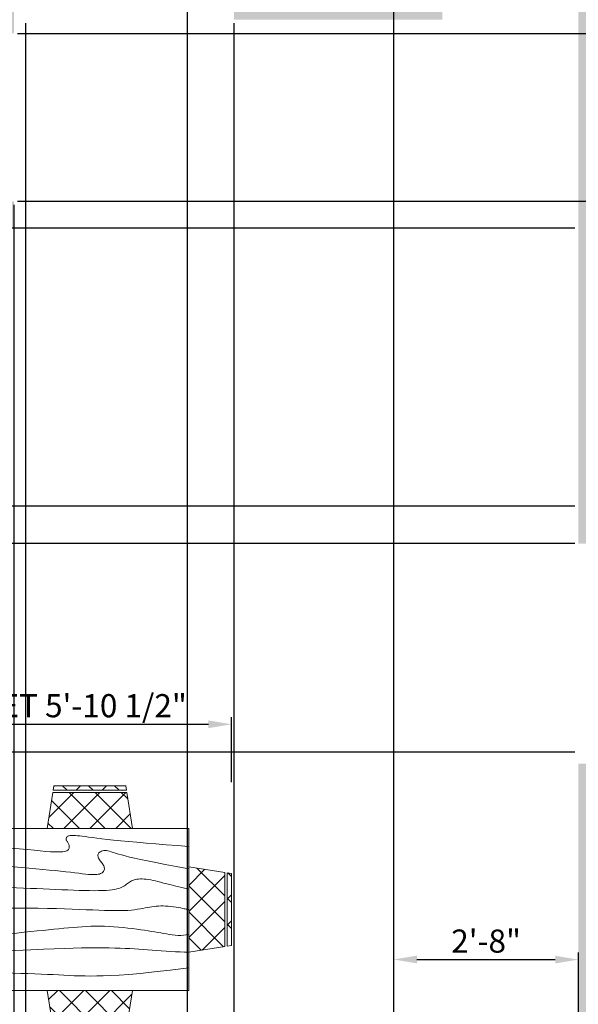
# Model space of a CAD drawing. Units: inches. Extents: x 1872 to 2380, y 714 to 1327.
# Tile 7 of 9: x 2101 to 2198, y 974 to 1144. Entities that reach past the tile are written whole.
import ezdxf

# ---------------------------------------------------------------- set-up
doc = ezdxf.new("R2010")
doc.units = ezdxf.units.IN
doc.layers.add('A-ANNO-DIMS', color=2, linetype='Continuous', lineweight=18)
doc.layers.add('A-FURN', color=8, linetype='Continuous', lineweight=18)
doc.layers.add('A-FURN-PATT', color=254, linetype='Continuous', lineweight=13, true_color=0xf8ceb3)
doc.layers.add('A-WALL-PATT', color=242, linetype='Continuous', lineweight=13, true_color=0xd52e31)
doc.styles.get("Standard").update_dxf_attribs({"font": 'arial.ttf'})
doc.dimstyles.new('ISO-25', dxfattribs={"dimtxt": 4, "dimasz": 4, "dimexe": 1.25, "dimexo": 0.625, "dimtad": 1, "dimdec": 0, "dimlunit": 3, "dimtxsty": 'Standard', "dimcen": 2.5, "dimadec": 0, "dimazin": 0, "dimtfac": 1, "dimtdec": 0, "dimtmove": 0, "dimatfit": 3, "dimfxl": 1, "dimarcsym": 0})

# ---------------------------------------------------------------- blocks, each defined once
blk = doc.blocks.new('Dining Set - 36 x 72 in.')
for p, q in [((-22, 27.5), (-22.1562, 26.50042)), ((-5.8416, 26.5), (-22.1534, 26.5)), ((-22, 27.5), (-6, 27.5)), ((-5.8437, 26.49966), (-6, 27.5)), ((6, 27.5), (5.8438, 26.50042)), ((22.1584, 26.5), (5.8466, 26.5)), ((6, 27.5), (22, 27.5)), ((22.1563, 26.49966), (22, 27.5)), ((-22.2343, 26.00059), (-23.4847, 17.99762)), ((-22.2304, 26), (-5.7608, 26)), ((-4.5152, 17.99762), (-5.7655, 25.99926)), ((5.7657, 26.00059), (4.5153, 17.99762)), ((5.7696, 26), (22.2392, 26)), ((23.4848, 17.99762), (22.2345, 25.99926)), ((36, 18), (-36, 18)), ((-36, 18), (-36, -18)), ((36, -18), (36, 18)), ((-44.0006, 8.23428), (-35.9976, 9.48474)), ((44.0006, 8.23428), (35.9976, 9.48474)), ((-45.5, 8), (-44.5004, 8.15617)), ((-45.5, 8), (-45.5, -8)), ((-44.5, -8.15843), (-44.5, 8.15338)), ((-44, 8.23041), (-44, -8.23915)), ((44, 8.23041), (44, -8.23915)), ((44.5, -8.15843), (44.5, 8.15338)), ((45.5, 8), (44.5005, 8.15617)), ((45.5, 8), (45.5, -8)), ((-44.4997, -8.15631), (-45.5, -8)), ((-35.9976, -9.48476), (-43.9993, -8.2345)), ((35.9976, -9.48476), (43.9993, -8.2345)), ((44.4997, -8.15631), (45.5, -8)), ((-36, -18), (36, -18)), ((-22.2343, -26.0006), (-23.4847, -17.99762)), ((-4.5152, -17.99762), (-5.7655, -25.99928)), ((5.7657, -26.0006), (4.5153, -17.99762)), ((23.4848, -17.99762), (22.2345, -25.99928)), ((-22.2304, -26), (-5.7608, -26)), ((5.7696, -26), (22.2392, -26)), ((-22, -27.5), (-22.1562, -26.50044)), ((-5.8416, -26.5), (-22.1534, -26.5)), ((-22, -27.5), (-6, -27.5)), ((-5.8437, -26.49967), (-6, -27.5)), ((6, -27.5), (5.8438, -26.50044)), ((22.1584, -26.5), (5.8466, -26.5)), ((6, -27.5), (22, -27.5)), ((22.1563, -26.49967), (22, -27.5))]:
    blk.add_line(p, q)
for points in [[(-36, 15), (-31.1772, 14.97754), (-26.8079, 14.91406), (-22.8538, 14.81543), (-19.276, 14.6875), (-16.0362, 14.53613), (-13.0957, 14.36718), (-10.4159, 14.18652), (-7.9583, 14), (-5.6904, 13.81315), (-3.6035, 13.63021), (-1.6954, 13.45508), (0.0365, 13.29166), (1.5945, 13.14388), (2.9811, 13.01562), (4.1988, 12.9108), (5.25, 12.83333), (6.1393, 12.78613), (6.8802, 12.76823), (7.4883, 12.77767), (7.9792, 12.8125), (8.3685, 12.87077), (8.6719, 12.95052), (8.9049, 13.0498), (9.0833, 13.16666), (9.2205, 13.29899), (9.3216, 13.44401), (9.3895, 13.59879), (9.4271, 13.76041), (9.4373, 13.92594), (9.4232, 14.09245), (9.3875, 14.257), (9.3333, 14.41666), (9.2638, 14.56917), (9.1836, 14.71484), (9.0975, 14.85465), (9.0104, 14.98958), (8.9272, 15.1206), (8.8529, 15.2487), (8.7922, 15.37483), (8.75, 15.5), (8.7305, 15.62467), (8.7344, 15.74739), (8.7617, 15.86621), (8.8125, 15.97916), (8.8867, 16.08431), (8.9844, 16.17968), (9.1055, 16.26334), (9.25, 16.33333), (9.4189, 16.38802), (9.6172, 16.42708), (9.8506, 16.45052), (10.125, 16.45833), (10.4463, 16.45052), (10.8203, 16.42708), (11.2529, 16.38802), (11.75, 16.33333), (12.3184, 16.26318), (12.9694, 16.17838), (13.7151, 16.07991), (14.5677, 15.96875), (15.5395, 15.84586), (16.6426, 15.71224), (17.8893, 15.56884), (19.2917, 15.41666), (20.859, 15.25667), (22.5879, 15.08984), (24.4721, 14.91715), (26.5052, 14.73958), (28.6809, 14.5581), (30.9929, 14.3737), (33.4347, 14.18733), (36, 14)], [(-36, 10), (-28.9766, 10.14274), (-23.1725, 10.20442), (-18.4241, 10.19775), (-14.5677, 10.13541), (-11.4399, 10.03011), (-8.877, 9.89453), (-6.7154, 9.74137), (-4.7917, 9.58333), (-2.9698, 9.43082), (-1.2246, 9.28515), (0.4415, 9.14534), (2.026, 9.01041), (3.5266, 8.87939), (4.9408, 8.7513), (6.266, 8.62516), (7.5, 8.5), (8.6411, 8.37549), (9.6914, 8.2539), (10.6538, 8.13818), (11.5312, 8.03125), (12.3267, 7.93603), (13.043, 7.85547), (13.6831, 7.79248), (14.25, 7.75), (14.7471, 7.7303), (15.1797, 7.73307), (15.5537, 7.75732), (15.875, 7.80208), (16.1494, 7.86637), (16.3828, 7.94922), (16.5811, 8.04964), (16.75, 8.16666), (16.8944, 8.29915), (17.0143, 8.44531), (17.1089, 8.60319), (17.1771, 8.77083), (17.218, 8.94629), (17.2305, 9.1276), (17.2137, 9.31282), (17.1667, 9.5), (17.0895, 9.6875), (16.987, 9.875), (16.8649, 10.0625), (16.7292, 10.25), (16.5856, 10.4375), (16.4401, 10.625), (16.2985, 10.8125), (16.1667, 11), (16.05, 11.18733), (15.9518, 11.3737), (15.8752, 11.5581), (15.8229, 11.73958), (15.798, 11.91715), (15.8034, 12.08984), (15.842, 12.25667), (15.9167, 12.41666), (16.0295, 12.56836), (16.1784, 12.70833), (16.3605, 12.83268), (16.5729, 12.9375), (16.8127, 13.01888), (17.0768, 13.07291), (17.3625, 13.0957), (17.6667, 13.08333), (17.9894, 13.03312), (18.3418, 12.94726), (18.7382, 12.82918), (19.1927, 12.68229), (19.7195, 12.51001), (20.3327, 12.31575), (21.0465, 12.10294), (21.875, 11.875), (22.8357, 11.63354), (23.959, 11.37304), (25.2786, 11.08618), (26.8282, 10.76562), (28.6414, 10.40405), (30.752, 9.99414), (33.1936, 9.52856), (36, 9)], [(-36, 5.5), (-30.7157, 5.3348), (-26.069, 5.20963), (-21.9946, 5.11767), (-18.4271, 5.05208), (-15.3009, 5.00602), (-12.5508, 4.97265), (-10.1112, 4.94515), (-7.9167, 4.91666), (-5.909, 4.88167), (-4.0586, 4.83984), (-2.3429, 4.79215), (-0.7396, 4.73958), (0.7739, 4.6831), (2.22, 4.6237), (3.6213, 4.56233), (5, 4.5), (6.373, 4.43782), (7.7344, 4.3776), (9.0723, 4.32129), (10.375, 4.27083), (11.6309, 4.22819), (12.8281, 4.19531), (13.9551, 4.17415), (15, 4.16666), (15.954, 4.17448), (16.819, 4.19791), (17.6001, 4.23698), (18.3021, 4.29166), (18.9299, 4.36198), (19.4883, 4.44791), (19.9823, 4.54948), (20.4167, 4.66666), (20.7969, 4.79899), (21.1302, 4.94401), (21.4245, 5.09879), (21.6875, 5.26041), (21.9271, 5.42594), (22.1511, 5.59245), (22.3672, 5.757), (22.5834, 5.91666), (22.8065, 6.06868), (23.0404, 6.21093), (23.2879, 6.34147), (23.5521, 6.45833), (23.8358, 6.55957), (24.142, 6.64323), (24.4735, 6.70735), (24.8334, 6.75), (25.2235, 6.76969), (25.642, 6.76692), (26.0858, 6.74267), (26.5521, 6.69791), (27.0379, 6.63362), (27.5404, 6.55078), (28.0565, 6.45036), (28.5834, 6.33333), (29.1242, 6.19987), (29.7071, 6.04687), (30.3661, 5.87044), (31.1354, 5.66666), (32.0493, 5.43164), (33.142, 5.16146), (34.4475, 4.85221), (36, 4.5)], [(-36, -1), (-30.7915, -0.6591), (-26.0195, -0.38216), (-21.6519, -0.16284), (-17.6563, 0.00521), (-14.0005, 0.12833), (-10.6523, 0.21289), (-7.5796, 0.26522), (-4.75, 0.29166), (-2.134, 0.29793), (0.2878, 0.28711), (2.5317, 0.26163), (4.6146, 0.22396), (6.5529, 0.17651), (8.3633, 0.12174), (10.0623, 0.06209), (11.6667, 0), (13.1899, -0.06201), (14.6341, -0.1211), (15.9982, -0.17432), (17.2813, -0.21875), (18.4823, -0.25147), (19.6003, -0.26953), (20.6343, -0.27002), (21.5834, -0.25), (22.4481, -0.20768), (23.2357, -0.14584), (23.9549, -0.06836), (24.6146, 0.02083), (25.2235, 0.11784), (25.7904, 0.21875), (26.3241, 0.31966), (26.8334, 0.41666), (27.3265, 0.50618), (27.8099, 0.58593), (28.2894, 0.65397), (28.7709, 0.70833), (29.2601, 0.74707), (29.763, 0.76823), (30.2855, 0.76985), (30.8334, 0.75), (31.4088, 0.70784), (31.9994, 0.64713), (32.589, 0.57275), (33.1615, 0.48958), (33.7008, 0.4025), (34.1908, 0.3164), (34.6153, 0.23616), (34.9584, 0.16666), (35.2099, 0.11165), (35.3848, 0.07031), (35.504, 0.04069), (35.5886, 0.02083), (35.6594, 0.00879), (35.7377, 0.0026), (35.8442, 0.00032), (36, 0)], [(-36, -6.5), (-27.1843, -6.31267), (-20.084, -6.1263), (-14.469, -5.9419), (-10.1094, -5.76042), (-6.7752, -5.58285), (-4.2363, -5.41016), (-2.2629, -5.24333), (-0.625, -5.08334), (0.8708, -4.93099), (2.2715, -4.78646), (3.5872, -4.64974), (4.8281, -4.52084), (6.0046, -4.39974), (7.127, -4.28646), (8.2053, -4.18099), (9.25, -4.08334), (10.2705, -3.99382), (11.2734, -3.91407), (12.2647, -3.84603), (13.25, -3.79167), (14.2354, -3.75293), (15.2266, -3.73177), (16.2295, -3.73015), (17.25, -3.75), (18.2912, -3.79248), (19.3451, -3.85547), (20.4009, -3.93604), (21.4479, -4.03125), (22.4754, -4.13819), (23.4727, -4.25391), (24.4289, -4.37549), (25.3334, -4.5), (26.1785, -4.62492), (26.9694, -4.74935), (27.7145, -4.87281), (28.4219, -4.99479), (29.1, -5.11483), (29.7572, -5.23242), (30.4016, -5.34709), (31.0417, -5.45834), (31.6837, -5.56437), (32.3262, -5.65821), (32.9658, -5.73153), (33.599, -5.77604), (34.2224, -5.78345), (34.8327, -5.74545), (35.4264, -5.65373), (36, -5.5)], [(-36, -10), (-26.4022, -9.81299), (-18.4675, -9.62891), (-11.9839, -9.45069), (-6.7396, -9.28125), (-2.5226, -9.12354), (0.8789, -8.98047), (3.6769, -8.85498), (6.0833, -8.75), (8.2767, -8.66765), (10.3021, -8.60677), (12.1712, -8.56543), (13.8958, -8.54167), (15.4876, -8.53353), (16.9583, -8.53907), (18.3197, -8.55632), (19.5834, -8.58334), (20.7616, -8.61841), (21.8685, -8.66081), (22.9188, -8.71004), (23.9271, -8.76563), (24.9081, -8.82707), (25.8763, -8.89388), (26.8465, -8.96558), (27.8334, -9.04167), (28.8474, -9.12118), (29.8828, -9.20117), (30.93, -9.27824), (31.9792, -9.34896), (33.0205, -9.40991), (34.0443, -9.45768), (35.0407, -9.48885), (36, -9.5)], [(-36, -14.5), (-30.0881, -14.33513), (-25.0332, -14.21224), (-20.7312, -14.12647), (-17.0781, -14.07292), (-13.97, -14.04671), (-11.3027, -14.04297), (-8.9724, -14.05681), (-6.875, -14.08334), (-4.9224, -14.11833), (-3.0905, -14.16016), (-1.3709, -14.20785), (0.2448, -14.26042), (1.7647, -14.3169), (3.1973, -14.3763), (4.5507, -14.43767), (5.8333, -14.5), (7.0554, -14.5621), (8.235, -14.62175), (9.3922, -14.67652), (10.5469, -14.72396), (11.7192, -14.76164), (12.929, -14.78711), (14.1965, -14.79794), (15.5417, -14.79167), (16.9933, -14.76424), (18.6152, -14.70508), (20.4804, -14.60197), (22.6615, -14.44271), (25.2312, -14.21509), (28.2624, -13.9069), (31.8277, -13.50594), (36, -13)]]:
    blk.add_lwpolyline(points)
blk = doc.blocks.new('*D46')
at = {"layer": 'A-ANNO-DIMS', "color": 0, "lineweight": -2, "transparency": 16777216}
for p, q in [((2067.28, 1012.46), (2067.28, 1023.69)), ((2071.28, 1022.44), (2133.99, 1022.44)), ((2137.99, 1012.46), (2137.99, 1023.69))]:
    blk.add_line(p, q, dxfattribs=at)
at = {"layer": 'A-ANNO-DIMS', "color": 0, "transparency": 16777216}
for points in [[(2071.28, 1023.11), (2071.28, 1021.77), (2067.28, 1022.44)], [(2133.99, 1023.11), (2133.99, 1021.77), (2137.99, 1022.44)]]:
    blk.add_solid(points, dxfattribs=at)
at = {"layer": 'Defpoints', "color": 0, "transparency": 16777216}
for p in [(2137.99, 1022.44), (2067.28, 1011.83), (2137.99, 1011.83)]:
    blk.add_point(p, dxfattribs=at)
at = {"layer": 'A-ANNO-DIMS', "color": 0, "transparency": 16777216, "insert": (2102.64, 1025.13), "char_height": 4, "attachment_point": 5}
blk.add_mtext('DINING SET 5\'-10 1/2"', dxfattribs=at)
blk = doc.blocks.new('*D69')
at = {"layer": 'A-ANNO-DIMS', "color": 0, "lineweight": -2, "transparency": 16777216}
for p, q in [((2101.02, 1141.77), (2377.6, 1141.77)), ((2376.35, 1116.77), (2376.35, 1137.77)), ((2101.02, 1112.77), (2377.6, 1112.77))]:
    blk.add_line(p, q, dxfattribs=at)
at = {"layer": 'A-ANNO-DIMS', "color": 0, "transparency": 16777216}
for points in [[(2375.68, 1137.77), (2377.01, 1137.77), (2376.35, 1141.77)], [(2375.68, 1116.77), (2377.01, 1116.77), (2376.35, 1112.77)]]:
    blk.add_solid(points, dxfattribs=at)
at = {"layer": 'Defpoints', "color": 0, "transparency": 16777216}
for p in [(2100.4, 1141.77), (2376.35, 1141.77), (2100.4, 1112.77)]:
    blk.add_point(p, dxfattribs=at)
at = {"layer": 'A-ANNO-DIMS', "color": 0, "transparency": 16777216, "insert": (2373.68, 1127.27), "char_height": 4, "attachment_point": 5, "rotation": 90}
blk.add_mtext('2\'-5"', dxfattribs=at)
blk = doc.blocks.new('*D70')
at = {"layer": 'A-ANNO-DIMS', "color": 0, "lineweight": -2, "transparency": 16777216}
for p, q in [((2102.4, 1143.52), (2102.4, 716.39)), ((2138.4, 1143.52), (2138.4, 716.39)), ((2106.4, 717.64), (2134.4, 717.64))]:
    blk.add_line(p, q, dxfattribs=at)
at = {"layer": 'A-ANNO-DIMS', "color": 0, "transparency": 16777216}
for points in [[(2106.4, 718.3), (2106.4, 716.97), (2102.4, 717.64)], [(2134.4, 718.3), (2134.4, 716.97), (2138.4, 717.64)]]:
    blk.add_solid(points, dxfattribs=at)
at = {"layer": 'Defpoints', "color": 0, "transparency": 16777216}
for p in [(2102.4, 1144.14), (2138.4, 1144.14), (2138.4, 717.64)]:
    blk.add_point(p, dxfattribs=at)
at = {"layer": 'A-ANNO-DIMS', "color": 0, "transparency": 16777216, "insert": (2120.4, 720.31), "char_height": 4, "attachment_point": 5}
blk.add_mtext('3\'-0"', dxfattribs=at)
blk = doc.blocks.new('*D72')
at = {"layer": 'A-ANNO-DIMS', "color": 0, "lineweight": -2, "transparency": 16777216}
for p, q in [((2197.27, 1108.14), (1905.35, 1108.14)), ((1906.6, 1064.14), (1906.6, 1104.14)), ((2197.27, 1060.14), (1905.35, 1060.14))]:
    blk.add_line(p, q, dxfattribs=at)
at = {"layer": 'A-ANNO-DIMS', "color": 0, "transparency": 16777216}
for points in [[(1905.93, 1104.14), (1907.27, 1104.14), (1906.6, 1108.14)], [(1905.93, 1064.14), (1907.27, 1064.14), (1906.6, 1060.14)]]:
    blk.add_solid(points, dxfattribs=at)
at = {"layer": 'Defpoints', "color": 0, "transparency": 16777216}
for p in [(1906.6, 1108.14), (2197.9, 1108.14), (2197.9, 1060.14)]:
    blk.add_point(p, dxfattribs=at)
at = {"layer": 'A-ANNO-DIMS', "color": 0, "transparency": 16777216, "insert": (1903.93, 1084.14), "char_height": 4, "attachment_point": 5, "rotation": 90}
blk.add_mtext('4\'-0"', dxfattribs=at)
blk = doc.blocks.new('*D73')
at = {"layer": 'A-ANNO-DIMS', "color": 0, "lineweight": -2, "transparency": 16777216}
for p, q in [((2197.27, 1053.64), (1905.35, 1053.64)), ((1906.6, 1021.64), (1906.6, 1049.64)), ((2197.27, 1017.64), (1905.35, 1017.64))]:
    blk.add_line(p, q, dxfattribs=at)
at = {"layer": 'A-ANNO-DIMS', "color": 0, "transparency": 16777216}
for points in [[(1905.93, 1049.64), (1907.27, 1049.64), (1906.6, 1053.64)], [(1905.93, 1021.64), (1907.27, 1021.64), (1906.6, 1017.64)]]:
    blk.add_solid(points, dxfattribs=at)
at = {"layer": 'Defpoints', "color": 0, "transparency": 16777216}
for p in [(1906.6, 1053.64), (2197.9, 1053.64), (2197.9, 1017.64)]:
    blk.add_point(p, dxfattribs=at)
at = {"layer": 'A-ANNO-DIMS', "color": 0, "transparency": 16777216, "insert": (1903.93, 1035.64), "char_height": 4, "attachment_point": 5, "rotation": 90}
blk.add_mtext('3\'-0"', dxfattribs=at)
blk = doc.blocks.new('*D74')
at = {"layer": 'A-ANNO-DIMS', "color": 0, "lineweight": -2, "transparency": 16777216}
for p, q in [((2130.4, 953.62), (2130.4, 1319.69)), ((2134.4, 1318.44), (2162.01, 1318.44)), ((2166.01, 953.64), (2166.01, 1319.69))]:
    blk.add_line(p, q, dxfattribs=at)
at = {"layer": 'A-ANNO-DIMS', "color": 0, "transparency": 16777216}
for points in [[(2134.4, 1319.11), (2134.4, 1317.78), (2130.4, 1318.44)], [(2162.01, 1319.11), (2162.01, 1317.78), (2166.01, 1318.44)]]:
    blk.add_solid(points, dxfattribs=at)
at = {"layer": 'Defpoints', "color": 0, "transparency": 16777216}
for p in [(2166.01, 1318.44), (2130.4, 952.99), (2166.01, 953.01)]:
    blk.add_point(p, dxfattribs=at)
at = {"layer": 'A-ANNO-DIMS', "color": 0, "transparency": 16777216, "insert": (2148.2, 1321.14), "char_height": 4, "attachment_point": 5}
blk.add_mtext('2\'-11 1/2"', dxfattribs=at)
blk = doc.blocks.new('*D75')
at = {"layer": 'A-ANNO-DIMS', "color": 0, "lineweight": -2, "transparency": 16777216}
for p, q in [((2166.01, 953.64), (2166.02, 983.06)), ((2197.9, 953.62), (2197.91, 983.04)), ((2170.02, 981.81), (2193.91, 981.8))]:
    blk.add_line(p, q, dxfattribs=at)
at = {"layer": 'A-ANNO-DIMS', "color": 0, "transparency": 16777216}
for points in [[(2170.02, 982.48), (2170.02, 981.14), (2166.02, 981.81)], [(2193.91, 982.46), (2193.91, 981.13), (2197.91, 981.79)]]:
    blk.add_solid(points, dxfattribs=at)
at = {"layer": 'Defpoints', "color": 0, "transparency": 16777216}
for p in [(2197.91, 981.79), (2166.01, 953.01), (2197.9, 952.99)]:
    blk.add_point(p, dxfattribs=at)
at = {"layer": 'A-ANNO-DIMS', "color": 0, "transparency": 16777216, "insert": (2181.97, 984.47), "char_height": 4, "attachment_point": 5, "rotation": 359.9714}
blk.add_mtext('2\'-8"', dxfattribs=at)
blk = doc.blocks.new('*D80')
at = {"layer": 'A-ANNO-DIMS', "color": 0, "lineweight": -2, "transparency": 16777216}
for p, q in [((2095.9, 1112.15), (2095.9, 716.39)), ((2100.4, 1112.15), (2100.4, 716.39)), ((2091.9, 717.64), (2087.9, 717.64)), ((2095.9, 717.64), (2100.4, 717.64)), ((2104.4, 717.64), (2129.6, 717.64))]:
    blk.add_line(p, q, dxfattribs=at)
at = {"layer": 'A-ANNO-DIMS', "color": 0, "transparency": 16777216}
for points in [[(2091.9, 718.3), (2091.9, 716.97), (2095.9, 717.64)], [(2104.4, 718.3), (2104.4, 716.97), (2100.4, 717.64)]]:
    blk.add_solid(points, dxfattribs=at)
at = {"layer": 'Defpoints', "color": 0, "transparency": 16777216}
for p in [(2095.9, 1112.77), (2100.4, 1112.77), (2100.4, 717.64)]:
    blk.add_point(p, dxfattribs=at)
at = {"layer": 'A-ANNO-DIMS', "color": 0, "transparency": 16777216, "insert": (2119, 720.33), "char_height": 4, "attachment_point": 5}
blk.add_mtext('0\'-4 1/2"', dxfattribs=at)

msp = doc.modelspace()

# ---------------------------------------------------------------- hatches: boundary and pattern name
at = {"layer": 'A-FURN-PATT', "transparency": 33554687}
h = msp.add_hatch(dxfattribs=at)
h.set_pattern_fill('ANSI37', color=256)
h.paths.add_polyline_path([(2030.37, 1262.04), (1979.97, 1262.04), (1979.97, 1246.84), (1967.17, 1246.84), (1967.17, 1202.04), (2030.37, 1202.04)])
h.paths.add_polyline_path([(1964.77, 1246.84), (1966.77, 1248.84), (1966.77, 1254.04), (1951.57, 1254.04), (1951.57, 1233.24), (1964.77, 1233.24)])
h.paths.add_polyline_path([(1964.77, 1230.84), (1951.57, 1230.84), (1951.57, 1210.04), (1964.77, 1210.04)])
h.paths.add_polyline_path([(2268.08, 1263.68), (2221.12, 1263.68), (2221.12, 1219.09), (2258.57, 1219.09), (2258.57, 1230.39), (2268.08, 1230.39)])
h.paths.add_polyline_path([(2279.67, 1257.73), (2269.86, 1257.73), (2269.86, 1242.28), (2279.67, 1242.28)])
h.paths.add_polyline_path([(2279.67, 1240.49), (2269.86, 1240.49), (2269.86, 1230.39), (2268.38, 1228.9), (2268.38, 1225.04), (2279.67, 1225.04)])
h.paths.add_polyline_path([(2097.97, 1011.83), (2085.54, 1011.83), (2085.42, 1011.06), (2098.09, 1011.06)])
h.paths.add_polyline_path([(2098.15, 1010.67), (2085.36, 1010.67), (2084.39, 1004.45), (2099.13, 1004.45)])
h.paths.add_polyline_path([(2119.91, 1010.67), (2107.12, 1010.67), (2106.14, 1004.45), (2120.89, 1004.45)])
h.paths.add_polyline_path([(2119.73, 1011.83), (2107.3, 1011.83), (2107.18, 1011.06), (2119.85, 1011.06)])
h.paths.add_polyline_path([(2074.66, 997.83), (2068.44, 996.86), (2068.44, 984.06), (2074.66, 983.09)])
h.paths.add_polyline_path([(2068.05, 996.8), (2067.28, 996.68), (2067.28, 984.25), (2068.05, 984.12)])
h.paths.add_polyline_path([(2136.83, 996.86), (2130.61, 997.83), (2130.61, 983.09), (2136.83, 984.06)])
h.paths.add_polyline_path([(2137.99, 996.68), (2137.22, 996.8), (2137.22, 984.12), (2137.99, 984.25)])
h.paths.add_polyline_path([(2099.13, 976.47), (2084.39, 976.47), (2085.36, 970.26), (2098.15, 970.26)])
h.paths.add_polyline_path([(2120.89, 976.47), (2106.14, 976.47), (2107.12, 970.26), (2119.91, 970.26)])
h.paths.add_polyline_path([(2119.85, 969.87), (2107.18, 969.87), (2107.3, 969.09), (2119.73, 969.09)])
h.paths.add_polyline_path([(2098.09, 969.87), (2085.42, 969.87), (2085.54, 969.09), (2097.97, 969.09)])
at = {"layer": 'A-WALL-PATT', "transparency": 33554687}
h = msp.add_hatch(color=256, dxfattribs=at)
h.dxf.hatch_style = 1
h.paths.add_polyline_path([(2295.4, 1289.64), (1935.4, 1289.64), (1935.4, 809.64), (1949.4, 809.64), (1949.4, 818.64), (1944.4, 818.64), (1944.4, 1108.27), (2100.4, 1108.27), (2100.4, 1112.77), (1944.4, 1112.77), (1944.4, 1280.64), (2095.9, 1280.64), (2095.9, 1141.77), (2100.4, 1141.77), (2100.4, 1280.64), (2169.91, 1280.64), (2169.91, 1244.64), (2169.91, 1160.49, -0.053008), (2170.04, 1158.75, -0.03687), (2169.91, 1157.54), (2169.91, 1148.64), (2167.91, 1148.64), (2138.4, 1148.64), (2138.4, 1144.14), (2167.91, 1144.14), (2174.41, 1144.14), (2174.41, 1280.64), (2197.9, 1280.64), (2197.9, 1184.64), (2202.4, 1184.64), (2202.4, 1280.64), (2286.4, 1280.64), (2286.4, 1148.64), (2197.9, 1148.64), (2197.9, 1108.14), (2202.4, 1108.14), (2202.4, 1144.14), (2286.4, 1144.14), (2286.4, 1060.14), (2202.4, 1060.14), (2202.4, 1108.14), (2197.9, 1108.14), (2197.9, 1060.14), (2197.9, 1053.64), (2202.4, 1053.64), (2202.4, 1055.64), (2286.4, 1055.64), (2286.4, 976.14), (2202.4, 976.14), (2202.4, 1015.64), (2197.9, 1015.64), (2197.9, 971.64), (2197.9, 952.99), (2197.9, 818.64), (2101.9, 818.64), (2101.9, 948.71), (2130.4, 948.71), (2130.4, 952.99), (2073.4, 952.99), (2073.4, 948.71), (2097.4, 948.71), (2097.4, 818.64), (2005.9, 818.64), (2005.9, 948.71), (2029.9, 948.71), (2029.9, 952.99), (2001.4, 952.99), (2001.4, 818.64), (1996.4, 818.64), (1985.23, 818.64), (1985.23, 809.64), (1996.4, 809.64), (2295.4, 809.64)])
h.paths.add_polyline_path([(2202.4, 971.64), (2286.4, 971.64), (2286.4, 858.19), (2286.62, 858.19), (2286.62, 857.19), (2286.4, 857.19), (2286.4, 828.68), (2286.48, 828.76), (2286.4, 828.43), (2286.4, 818.64), (2256.29, 818.64), (2255.29, 818.39), (2254.54, 818.64), (2238.99, 818.64), (2238.75, 818.58), (2238.56, 818.64), (2202.4, 818.64), (2202.4, 952.99)], flags=16)
h.paths.add_polyline_path([(2260.41, 970, -0.15), (2280.41, 970), (2278.41, 967, 0.001913), (2277.92, 967.06), (2277.41, 964.5), (2278.64, 964.5), (2278.72, 964), (2279.41, 964), (2282.41, 953, -0.541163), (2280.76, 950.93), (2280.91, 950, -0.414214), (2279.91, 949), (2279.41, 949), (2279.91, 945), (2278.41, 945), (2277.91, 949), (2270.41, 949), (2262.91, 949), (2262.41, 945), (2260.91, 945), (2261.41, 949), (2260.91, 949, -0.414214), (2259.91, 950), (2260.05, 950.93, -0.505809), (2258.36, 952.83), (2261.41, 964), (2262.1, 964), (2262.17, 964.5), (2263.41, 964.5), (2262.9, 967.06, 0.001913), (2262.41, 967)], flags=0)
h.paths.add_polyline_path([(2257.85, 934.42), (2280.51, 934.42, -0.333333), (2281.77, 933.16), (2281.77, 923.09, -0.333333), (2280.51, 921.83), (2277.57, 921.83), (2277.57, 921.41), (2275.89, 921.41), (2275.89, 921.83), (2262.46, 921.83), (2262.46, 921.41), (2260.79, 921.41), (2260.79, 921.83), (2257.85, 921.83, -0.333333), (2256.59, 923.09), (2256.59, 933.16, -0.333333)], flags=0)
h.paths.add_polyline_path([(2260.61, 912.79), (2262.11, 912.79), (2262.61, 908.79), (2270.11, 908.79), (2277.61, 908.79), (2278.11, 912.79), (2279.61, 912.79), (2279.11, 908.79), (2279.61, 908.79, -0.414214), (2280.61, 907.79), (2280.46, 906.86, -0.505809), (2282.15, 904.96), (2279.11, 893.79), (2278.42, 893.79), (2278.34, 893.29), (2277.11, 893.29), (2277.62, 890.73, 0.001913), (2278.11, 890.79), (2280.11, 887.79, -0.15), (2260.11, 887.79), (2262.11, 890.79, 0.001913), (2262.59, 890.73), (2263.11, 893.29), (2261.87, 893.29), (2261.79, 893.79), (2261.11, 893.79), (2258.11, 904.79, -0.541163), (2259.75, 906.86), (2259.61, 907.79, -0.414214), (2260.61, 908.79), (2261.11, 908.79)], flags=0)
h.paths.add_polyline_path([(2252.62, 864.69), (2253.62, 864.69), (2253.62, 862.19), (2253.62, 860.69), (2256.62, 859.69, -0.362186), (2259.62, 862.19, -0.174416), (2262.62, 860.69, 0.103487), (2265.62, 859.19, -0.219276), (2266.55, 858.19), (2268.62, 858.19), (2268.62, 859.69), (2267.62, 859.69), (2267.62, 863.69), (2270.12, 863.69), (2270.12, 859.69), (2269.12, 859.69), (2269.12, 858.19), (2274.62, 858.19), (2278.62, 858.19), (2278.62, 862.69), (2275.62, 864.69), (2275.62, 865.69), (2279.62, 862.69), (2279.62, 858.19), (2279.62, 852.69), (2275.62, 849.19), (2275.62, 850.19), (2278.62, 852.69), (2278.62, 857.19), (2274.62, 857.19), (2271.12, 857.19), (2271.12, 855.69), (2272.12, 855.69), (2272.12, 851.69), (2269.62, 851.69), (2269.62, 855.69), (2270.62, 855.69), (2270.62, 857.19), (2266.55, 857.19, -0.219162), (2265.62, 856.19, 0.103506), (2262.62, 854.69, -0.174459), (2259.62, 853.19, -0.362114), (2256.62, 855.69), (2253.62, 854.69), (2253.62, 850.69), (2252.62, 850.69)], flags=0)
h.paths.add_polyline_path([(2253.62, 859.69), (2256.62, 858.69), (2256.62, 856.69), (2253.62, 855.69)], flags=0)
h.paths.add_polyline_path([(2208.62, 838.17), (2208.28, 836.61), (2207.75, 836.18), (2207.67, 833.93), (2208.71, 832.96), (2211.55, 836.09), (2214.43, 837.53), (2214.45, 837.55), (2214.61, 836.16), (2215.48, 834.9), (2215.87, 835.13), (2217.12, 836.79), (2216.83, 834.17), (2218.8, 828.76), (2219.23, 829.13), (2220.06, 831.53), (2219.5, 837.61), (2219.53, 837.66), (2219.68, 838.72), (2219.62, 838.91), (2219.72, 839.01), (2219.51, 837.47), (2219.77, 834.68), (2220.87, 834.05), (2221.03, 834.58), (2222.05, 835.47), (2222.71, 834.65), (2223.67, 836.89), (2224.63, 836.57), (2226.23, 835.08), (2227.55, 836.18), (2227.59, 837.16), (2228.42, 838.17), (2228.08, 836.61), (2227.55, 836.18), (2227.47, 833.93), (2228.51, 832.96), (2231.35, 836.09), (2234.23, 837.53), (2234.25, 837.55), (2234.42, 836.16), (2235.28, 834.9), (2235.67, 835.13), (2236.93, 836.79), (2236.93, 836.84), (2238.69, 834.65), (2239.41, 836.34), (2239.3, 837.61), (2239.34, 837.66), (2239.48, 838.72), (2239.42, 838.91), (2239.52, 839.01), (2239.31, 837.47), (2239.36, 836.98), (2240.61, 836.57), (2242.2, 835.08), (2243.53, 836.18), (2243.57, 837.16), (2244.39, 838.17), (2244.05, 836.61), (2243.53, 836.18), (2243.44, 833.93), (2244.49, 832.96), (2247.33, 836.09), (2250.21, 837.53), (2250.22, 837.55), (2250.39, 836.16), (2251.25, 834.9), (2251.65, 835.13), (2252.9, 836.79), (2252.61, 834.17), (2254.09, 830.08), (2254.54, 829.37), (2254.85, 828.99), (2255.01, 829.13), (2255.83, 831.53), (2255.29, 837.44), (2255.28, 837.44), (2255.46, 838.72), (2255.4, 838.91), (2255.5, 839.01), (2255.28, 837.47), (2255.29, 837.44), (2257.9, 836.57), (2259.5, 835.08), (2260.82, 836.18), (2260.86, 837.16), (2261.69, 838.17), (2261.35, 836.61), (2260.82, 836.18), (2260.74, 833.93), (2261.78, 832.96), (2264.62, 836.09), (2267.5, 837.53), (2267.52, 837.55), (2267.68, 836.16), (2268.54, 834.9), (2268.94, 835.13), (2270.19, 836.79), (2269.9, 834.17), (2271.79, 828.96), (2271.98, 828.86), (2272.3, 829.13), (2273.13, 831.53), (2272.56, 837.61), (2272.6, 837.66), (2272.75, 838.72), (2272.69, 838.91), (2272.79, 839.01), (2272.58, 837.47), (2273.13, 831.53), (2273.02, 831.22), (2273.67, 831.01), (2273.92, 831.6), (2273.83, 830.95), (2274.1, 830.86), (2275.75, 833.35), (2276.03, 831.86), (2276.57, 831.38), (2277, 831.91), (2277.3, 833.27), (2279.06, 830.44), (2281.09, 831.46), (2281.1, 831.48), (2281.21, 830.5), (2281.82, 829.61), (2282.1, 829.77), (2282.98, 830.94), (2282.77, 829.1), (2284.15, 825.3), (2284.46, 825.55), (2285.04, 827.24), (2284.64, 831.51), (2284.67, 831.55), (2284.77, 832.3), (2284.73, 832.43), (2284.8, 832.5), (2284.65, 831.42), (2285.04, 827.24), (2284.46, 825.55), (2283.45, 824.71), (2281.76, 819.99), (2278.73, 818.64), (2276.7, 819.65), (2275.69, 821.34), (2274.34, 822.01), (2272.32, 824.04), (2269.58, 824.33), (2268.46, 821.21), (2264.14, 819.29), (2261.26, 820.73), (2259.82, 823.13), (2257.9, 824.09), (2255.02, 826.97), (2253.29, 827.15), (2251.17, 821.21), (2246.85, 819.29), (2243.97, 820.73), (2242.53, 823.13), (2240.61, 824.09), (2237.73, 826.97), (2237.27, 827.01), (2235.19, 821.21), (2230.87, 819.29), (2227.99, 820.73), (2226.55, 823.13), (2224.63, 824.09), (2221.75, 826.97), (2217.61, 827.41), (2215.39, 821.21), (2211.07, 819.29), (2208.19, 820.73), (2206.75, 823.13), (2204.83, 824.09), (2203.87, 826.49), (2202.91, 830.81), (2202.91, 834.65), (2203.87, 836.89), (2204.83, 836.57), (2206.43, 835.08), (2207.75, 836.18), (2207.79, 837.16)], flags=0)
h.paths.add_polyline_path([(2221.04, 832.88), (2221.82, 832.52), (2222.11, 833.69), (2222.71, 834.29), (2222.71, 832.11), (2225.59, 830.81), (2226.55, 830.81), (2228.95, 822.65), (2230.87, 820.25), (2230.87, 819.29), (2233.27, 821.21), (2233.75, 823.61), (2232.79, 826.97), (2231.99, 830.19), (2236.41, 827.71), (2236.63, 831.29), (2235.93, 834.58), (2242.53, 830.81), (2241.57, 830.81), (2240.97, 831.07), (2240.47, 830.33), (2239.06, 829.14), (2239.65, 826.49), (2237.25, 829.37), (2236.52, 829.55), (2236.41, 827.71), (2231.99, 830.19), (2232.79, 826.97), (2233.75, 823.61), (2233.27, 821.21), (2230.87, 819.29), (2230.87, 820.25), (2228.95, 822.65), (2226.55, 830.81), (2225.59, 830.81), (2222.71, 832.11), (2222.71, 830.81), (2223.67, 826.49), (2221.27, 829.37), (2220.67, 830.33), (2220.67, 830.33)], flags=0)
h.paths.add_polyline_path([(2255.98, 833), (2259.82, 830.81), (2258.86, 830.81), (2257.25, 831.54), (2256.45, 830.33), (2256.66, 831.81), (2256.02, 832.1), (2255.98, 831.99)], flags=0)
h.paths.add_polyline_path([(2275.69, 826.73), (2277.07, 828.25), (2275.46, 829.74), (2276.39, 830.51), (2276.33, 828.93), (2279.06, 826.4), (2278.73, 823.36), (2277.38, 821)], flags=0)
h.paths.add_polyline_path([(2260.6, 925.25), (2276.34, 925.25), (2276.34, 931.01), (2260.6, 931.01)], flags=8)
h.paths.add_polyline_path([(2202.72, 1070.05), (2202.72, 1092.72), (2197.34, 1092.72), (2197.34, 1070.05)], flags=25)

# ---------------------------------------------------------------- block references
at = {"layer": 'A-FURN', "transparency": 33554687, "xscale": 0.7771303306467578, "yscale": 0.7771303306467578, "zscale": 0.7771303306467578}
msp.add_blockref('Dining Set - 36 x 72 in.', (2102.64, 990.46), dxfattribs=at)

# ---------------------------------------------------------------- dimensions: what is measured, and where the dimension line sits
at = {"layer": 'A-ANNO-DIMS', "transparency": 33554687}
for base, p1, p2, picture, middle in [((2166.01, 1318.44), (2130.4, 952.99), (2166.01, 953.01), '*D74', (2148.2, 1321.14)), ((2138.4, 717.64), (2102.4, 1144.14), (2138.4, 1144.14), '*D70', (2120.4, 720.31)), ((2100.4, 717.64), (2095.9, 1112.77), (2100.4, 1112.77), '*D80', (2119, 720.33))]:
    dim = msp.add_linear_dim(base=base, p1=p1, p2=p2, dimstyle='ISO-25', override={"dimdec": 1, "dimlfac": 1, "dimrnd": 0, "dimzin": 1, "dimdsep": 46, "dimlunit": 4, "dimfrac": 2}, dxfattribs=at)
    dim.commit()
    dim.dimension.update_dxf_attribs({"geometry": picture, "text_midpoint": middle})
for base, p1, p2, angle, picture, middle in [((2376.35, 1141.77), (2100.4, 1112.77), (2100.4, 1141.77), 90, '*D69', (2373.68, 1127.27)), ((1906.6, 1108.14), (2197.9, 1060.14), (2197.9, 1108.14), 90, '*D72', (1903.93, 1084.14)), ((1906.6, 1053.64), (2197.9, 1017.64), (2197.9, 1053.64), 90, '*D73', (1903.93, 1035.64)), ((2197.91, 981.79), (2166.01, 953.01), (2197.9, 952.99), 359.9714, '*D75', (2181.97, 984.47))]:
    dim = msp.add_linear_dim(base=base, p1=p1, p2=p2, angle=angle, dimstyle='ISO-25', override={"dimdec": 1, "dimlfac": 1, "dimrnd": 0, "dimzin": 1, "dimdsep": 46, "dimlunit": 4, "dimfrac": 2}, dxfattribs=at)
    dim.commit()
    dim.dimension.update_dxf_attribs({"geometry": picture, "text_midpoint": middle})
dim = msp.add_linear_dim(base=(2137.99, 1022.44), p1=(2067.28, 1011.83), p2=(2137.99, 1011.83), text='DINING SET <>', dimstyle='ISO-25', override={"dimdec": 1, "dimlfac": 1, "dimrnd": 0, "dimzin": 1, "dimdsep": 46, "dimlunit": 4, "dimfrac": 2}, dxfattribs=at)
dim.commit()
dim.dimension.update_dxf_attribs({"geometry": '*D46', "text_midpoint": (2102.64, 1025.13)})

doc.saveas('drawing.dxf')
